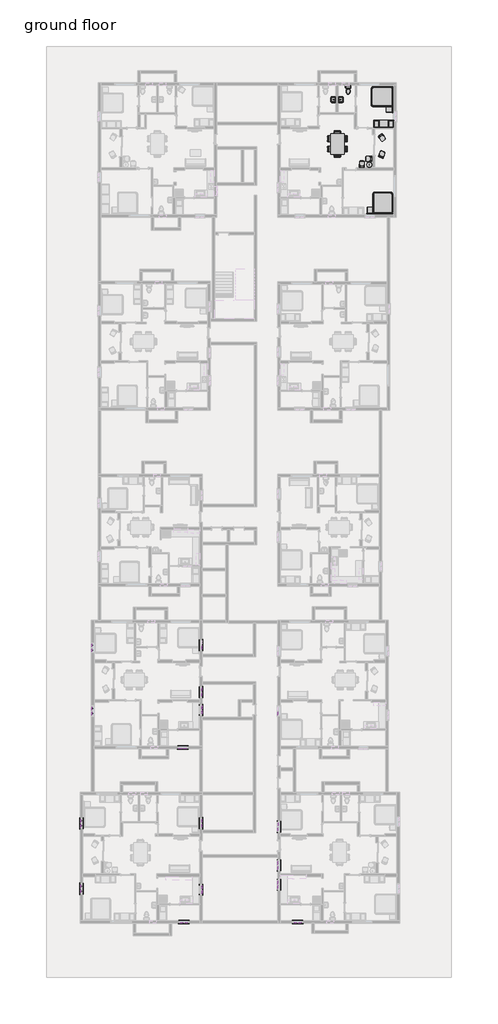
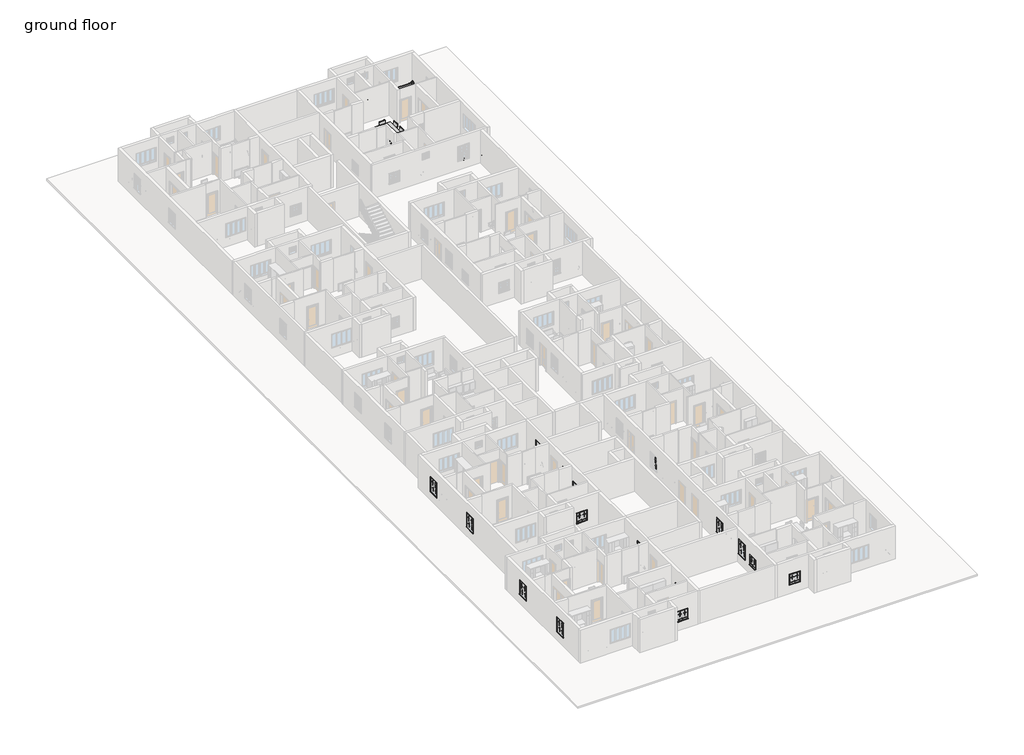
# One storey, part 14 of 16: 84 proxies, 15 furniture elements, 3 flow terminals.
"""IFC4 building model written with IfcOpenShell, lengths in millimetres."""

from ifc_helpers import new_model, si_unit, origin, place, context, project, spatial, transform, mapped, element, save
from components import muntin_pattern_2x2_muntin_pattern_2x2_cd1db81d, muntin_pattern_2x2_muntin_pattern_2x2_7c797e2d, muntin_pattern_2x2_muntin_pattern_2x2_78ce0566, muntin_pattern_2x2_muntin_pattern_2x2_27bf4e5b, muntin_pattern_2x2_muntin_pattern_2x2_8320156c, trim_window_exterior_flat_with_sill_fadbc092, trim_window_exterior_flat_with_sill_41619996, trim_window_interior_flat_picture_frame_db6fc9b7, trim_window_interior_flat_picture_frame_51c85655, flow_terminal_8d9ea526, toilet_domestic_3d_toilet_domestic_3d_ba6479b0, toilet_domestic_3d_toilet_domestic_3d_30431060, bed_design_8999_bed_design_8999_9c973422, bed_design_8999_bed_design_8999_e911dec7, chair_task_chair_task_b7f3823b, chair_task_arms_chair_task_arms_fa5a08ef, furniture_88072bd9, furniture_4fdbbe14, furniture_0bcc43ae, furniture_3dd5e188

model = new_model("IFC4")

# Units and contexts
model_context = context("Model", 3, world=origin())
ifc_project = project(units=[si_unit("LENGTHUNIT", "METRE", prefix="MILLI")], contexts=[model_context])

# Site, building, storey
site = spatial("IfcSite", under=ifc_project)
building = spatial("IfcBuilding", under=site)
storey = spatial("IfcBuildingStorey", under=building, Name="ground floor", Elevation=609.6)

# Proxies
placement = place(None, origin())
muntin_pattern_2x2_muntin_pattern_2x2_shape = muntin_pattern_2x2_muntin_pattern_2x2_cd1db81d(model_context)
element("IfcBuildingElementProxy", 1, Name="Muntin Pattern_2x2 : Muntin Pattern_2x2", ObjectType="Muntin Pattern_2x2 : Muntin Pattern_2x2", at=placement, inside=storey, context=model_context, shape_type="MappedRepresentation", body=[
    mapped(muntin_pattern_2x2_muntin_pattern_2x2_shape, transform((41563.651243, -22010.1303409, 2206.625), x_axis=(0.0, 1.0, 0.0), y_axis=(-1.0, 0.0, 0.0), z_axis=(0.0, 0.0, 1.0))),
])
element("IfcBuildingElementProxy", 2, Name="Muntin Pattern_2x2 : Muntin Pattern_2x2", ObjectType="Muntin Pattern_2x2 : Muntin Pattern_2x2", at=placement, inside=storey, context=model_context, shape_type="MappedRepresentation", body=[
    mapped(muntin_pattern_2x2_muntin_pattern_2x2_shape, transform((41608.101243, -22010.1303409, 1600.2), x_axis=(0.0, 1.0, 0.0), y_axis=(-1.0, 0.0, 0.0), z_axis=(0.0, 0.0, 1.0))),
])
element("IfcBuildingElementProxy", 3, Name="Muntin Pattern_2x2 : Muntin Pattern_2x2", ObjectType="Muntin Pattern_2x2 : Muntin Pattern_2x2", at=placement, inside=storey, context=model_context, shape_type="MappedRepresentation", body=[
    mapped(muntin_pattern_2x2_muntin_pattern_2x2_shape, transform((41563.651243, -16104.6303409, 2206.625), x_axis=(0.0, 1.0, 0.0), y_axis=(-1.0, 0.0, 0.0), z_axis=(0.0, 0.0, 1.0))),
])
element("IfcBuildingElementProxy", 4, Name="Muntin Pattern_2x2 : Muntin Pattern_2x2", ObjectType="Muntin Pattern_2x2 : Muntin Pattern_2x2", at=placement, inside=storey, context=model_context, shape_type="MappedRepresentation", body=[
    mapped(muntin_pattern_2x2_muntin_pattern_2x2_shape, transform((41608.101243, -16104.6303409, 1600.2), x_axis=(0.0, 1.0, 0.0), y_axis=(-1.0, 0.0, 0.0), z_axis=(0.0, 0.0, 1.0))),
])
element("IfcBuildingElementProxy", 5, Name="Muntin Pattern_2x2 : Muntin Pattern_2x2", ObjectType="Muntin Pattern_2x2 : Muntin Pattern_2x2", at=placement, inside=storey, context=model_context, shape_type="MappedRepresentation", body=[
    mapped(muntin_pattern_2x2_muntin_pattern_2x2_shape, transform((52504.701243, -16549.6721711, 2206.625), x_axis=(0.0, -1.0, 0.0), y_axis=(1.0, 0.0, 0.0), z_axis=(0.0, 0.0, 1.0))),
])
element("IfcBuildingElementProxy", 6, Name="Muntin Pattern_2x2 : Muntin Pattern_2x2", ObjectType="Muntin Pattern_2x2 : Muntin Pattern_2x2", at=placement, inside=storey, context=model_context, shape_type="MappedRepresentation", body=[
    mapped(muntin_pattern_2x2_muntin_pattern_2x2_shape, transform((52460.251243, -16549.6721711, 1600.2), x_axis=(0.0, -1.0, 0.0), y_axis=(1.0, 0.0, 0.0), z_axis=(0.0, 0.0, 1.0))),
])
element("IfcBuildingElementProxy", 7, Name="Muntin Pattern_2x2 : Muntin Pattern_2x2", ObjectType="Muntin Pattern_2x2 : Muntin Pattern_2x2", at=placement, inside=storey, context=model_context, shape_type="MappedRepresentation", body=[
    mapped(muntin_pattern_2x2_muntin_pattern_2x2_shape, transform((59391.4562819, -16409.4303409, 2206.625), x_axis=(0.0, 1.0, 0.0), y_axis=(-1.0, 0.0, 0.0), z_axis=(0.0, 0.0, 1.0))),
])
element("IfcBuildingElementProxy", 8, Name="Muntin Pattern_2x2 : Muntin Pattern_2x2", ObjectType="Muntin Pattern_2x2 : Muntin Pattern_2x2", at=placement, inside=storey, context=model_context, shape_type="MappedRepresentation", body=[
    mapped(muntin_pattern_2x2_muntin_pattern_2x2_shape, transform((59435.9062819, -16409.4303409, 1600.2), x_axis=(0.0, 1.0, 0.0), y_axis=(-1.0, 0.0, 0.0), z_axis=(0.0, 0.0, 1.0))),
])
element("IfcBuildingElementProxy", 9, Name="Muntin Pattern_2x2 : Muntin Pattern_2x2", ObjectType="Muntin Pattern_2x2 : Muntin Pattern_2x2", at=placement, inside=storey, context=model_context, shape_type="MappedRepresentation", body=[
    mapped(muntin_pattern_2x2_muntin_pattern_2x2_shape, transform((42566.951243, -5948.3051164, 2206.625), x_axis=(0.0, 1.0, 0.0), y_axis=(-1.0, 0.0, 0.0), z_axis=(0.0, 0.0, 1.0))),
])
element("IfcBuildingElementProxy", 10, Name="Muntin Pattern_2x2 : Muntin Pattern_2x2", ObjectType="Muntin Pattern_2x2 : Muntin Pattern_2x2", at=placement, inside=storey, context=model_context, shape_type="MappedRepresentation", body=[
    mapped(muntin_pattern_2x2_muntin_pattern_2x2_shape, transform((42611.401243, -5948.3051164, 1600.2), x_axis=(0.0, 1.0, 0.0), y_axis=(-1.0, 0.0, 0.0), z_axis=(0.0, 0.0, 1.0))),
])
element("IfcBuildingElementProxy", 11, Name="Muntin Pattern_2x2 : Muntin Pattern_2x2", ObjectType="Muntin Pattern_2x2 : Muntin Pattern_2x2", at=placement, inside=storey, context=model_context, shape_type="MappedRepresentation", body=[
    mapped(muntin_pattern_2x2_muntin_pattern_2x2_shape, transform((42566.951243, -233.3051164, 2206.625), x_axis=(0.0, 1.0, 0.0), y_axis=(-1.0, 0.0, 0.0), z_axis=(0.0, 0.0, 1.0))),
])
element("IfcBuildingElementProxy", 12, Name="Muntin Pattern_2x2 : Muntin Pattern_2x2", ObjectType="Muntin Pattern_2x2 : Muntin Pattern_2x2", at=placement, inside=storey, context=model_context, shape_type="MappedRepresentation", body=[
    mapped(muntin_pattern_2x2_muntin_pattern_2x2_shape, transform((42611.401243, -233.3051164, 1600.2), x_axis=(0.0, 1.0, 0.0), y_axis=(-1.0, 0.0, 0.0), z_axis=(0.0, 0.0, 1.0))),
])
element("IfcBuildingElementProxy", 13, Name="Muntin Pattern_2x2 : Muntin Pattern_2x2", ObjectType="Muntin Pattern_2x2 : Muntin Pattern_2x2", at=placement, inside=storey, context=model_context, shape_type="MappedRepresentation", body=[
    mapped(muntin_pattern_2x2_muntin_pattern_2x2_shape, transform((59391.4562819, -19899.7596399, 2206.625), x_axis=(0.0, 1.0, 0.0), y_axis=(-1.0, 0.0, 0.0), z_axis=(0.0, 0.0, 1.0))),
])
element("IfcBuildingElementProxy", 14, Name="Muntin Pattern_2x2 : Muntin Pattern_2x2", ObjectType="Muntin Pattern_2x2 : Muntin Pattern_2x2", at=placement, inside=storey, context=model_context, shape_type="MappedRepresentation", body=[
    mapped(muntin_pattern_2x2_muntin_pattern_2x2_shape, transform((59435.9062819, -19899.7596399, 1600.2), x_axis=(0.0, 1.0, 0.0), y_axis=(-1.0, 0.0, 0.0), z_axis=(0.0, 0.0, 1.0))),
])
element("IfcBuildingElementProxy", 15, Name="Muntin Pattern_2x2 : Muntin Pattern_2x2", ObjectType="Muntin Pattern_2x2 : Muntin Pattern_2x2", at=placement, inside=storey, context=model_context, shape_type="MappedRepresentation", body=[
    mapped(muntin_pattern_2x2_muntin_pattern_2x2_shape, transform((52504.701243, -4691.5814238, 2206.625), x_axis=(0.0, -1.0, 0.0), y_axis=(1.0, 0.0, 0.0), z_axis=(0.0, 0.0, 1.0))),
])
element("IfcBuildingElementProxy", 16, Name="Muntin Pattern_2x2 : Muntin Pattern_2x2", ObjectType="Muntin Pattern_2x2 : Muntin Pattern_2x2", at=placement, inside=storey, context=model_context, shape_type="MappedRepresentation", body=[
    mapped(muntin_pattern_2x2_muntin_pattern_2x2_shape, transform((52460.251243, -4691.5814238, 1600.2), x_axis=(0.0, -1.0, 0.0), y_axis=(1.0, 0.0, 0.0), z_axis=(0.0, 0.0, 1.0))),
])
element("IfcBuildingElementProxy", 17, Name="Muntin Pattern_2x2 : Muntin Pattern_2x2", ObjectType="Muntin Pattern_2x2 : Muntin Pattern_2x2", at=placement, inside=storey, context=model_context, shape_type="MappedRepresentation", body=[
    mapped(muntin_pattern_2x2_muntin_pattern_2x2_shape, transform((52504.701243, -452.6471815, 2206.625), x_axis=(0.0, -1.0, 0.0), y_axis=(1.0, 0.0, 0.0), z_axis=(0.0, 0.0, 1.0))),
])
element("IfcBuildingElementProxy", 18, Name="Muntin Pattern_2x2 : Muntin Pattern_2x2", ObjectType="Muntin Pattern_2x2 : Muntin Pattern_2x2", at=placement, inside=storey, context=model_context, shape_type="MappedRepresentation", body=[
    mapped(muntin_pattern_2x2_muntin_pattern_2x2_shape, transform((52460.251243, -452.6471815, 1600.2), x_axis=(0.0, -1.0, 0.0), y_axis=(1.0, 0.0, 0.0), z_axis=(0.0, 0.0, 1.0))),
])
muntin_pattern_2x2_muntin_pattern_2x2_2_shape = muntin_pattern_2x2_muntin_pattern_2x2_7c797e2d(model_context)
element("IfcBuildingElementProxy", 19, Name="Muntin Pattern_2x2 : Muntin Pattern_2x2", ObjectType="Muntin Pattern_2x2 : Muntin Pattern_2x2", at=placement, inside=storey, context=model_context, shape_type="MappedRepresentation", body=[
    mapped(muntin_pattern_2x2_muntin_pattern_2x2_2_shape, transform((59391.4562819, -6403.9176164, 2206.625), x_axis=(0.0, -1.0, 0.0), y_axis=(1.0, 0.0, 0.0), z_axis=(0.0, 0.0, 1.0))),
])
element("IfcBuildingElementProxy", 20, Name="Muntin Pattern_2x2 : Muntin Pattern_2x2", ObjectType="Muntin Pattern_2x2 : Muntin Pattern_2x2", at=placement, inside=storey, context=model_context, shape_type="MappedRepresentation", body=[
    mapped(muntin_pattern_2x2_muntin_pattern_2x2_2_shape, transform((59435.9062819, -6403.9176164, 1600.2), x_axis=(0.0, -1.0, 0.0), y_axis=(1.0, 0.0, 0.0), z_axis=(0.0, 0.0, 1.0))),
])
element("IfcBuildingElementProxy", 21, Name="Muntin Pattern_2x2 : Muntin Pattern_2x2", ObjectType="Muntin Pattern_2x2 : Muntin Pattern_2x2", at=placement, inside=storey, context=model_context, shape_type="MappedRepresentation", body=[
    mapped(muntin_pattern_2x2_muntin_pattern_2x2_2_shape, transform((41563.651243, -22465.7428409, 2206.625), x_axis=(0.0, -1.0, 0.0), y_axis=(1.0, 0.0, 0.0), z_axis=(0.0, 0.0, 1.0))),
])
element("IfcBuildingElementProxy", 22, Name="Muntin Pattern_2x2 : Muntin Pattern_2x2", ObjectType="Muntin Pattern_2x2 : Muntin Pattern_2x2", at=placement, inside=storey, context=model_context, shape_type="MappedRepresentation", body=[
    mapped(muntin_pattern_2x2_muntin_pattern_2x2_2_shape, transform((41608.101243, -22465.7428409, 1600.2), x_axis=(0.0, -1.0, 0.0), y_axis=(1.0, 0.0, 0.0), z_axis=(0.0, 0.0, 1.0))),
])
element("IfcBuildingElementProxy", 23, Name="Muntin Pattern_2x2 : Muntin Pattern_2x2", ObjectType="Muntin Pattern_2x2 : Muntin Pattern_2x2", at=placement, inside=storey, context=model_context, shape_type="MappedRepresentation", body=[
    mapped(muntin_pattern_2x2_muntin_pattern_2x2_2_shape, transform((41563.651243, -16560.2428409, 2206.625), x_axis=(0.0, -1.0, 0.0), y_axis=(1.0, 0.0, 0.0), z_axis=(0.0, 0.0, 1.0))),
])
element("IfcBuildingElementProxy", 24, Name="Muntin Pattern_2x2 : Muntin Pattern_2x2", ObjectType="Muntin Pattern_2x2 : Muntin Pattern_2x2", at=placement, inside=storey, context=model_context, shape_type="MappedRepresentation", body=[
    mapped(muntin_pattern_2x2_muntin_pattern_2x2_2_shape, transform((41608.101243, -16560.2428409, 1600.2), x_axis=(0.0, -1.0, 0.0), y_axis=(1.0, 0.0, 0.0), z_axis=(0.0, 0.0, 1.0))),
])
element("IfcBuildingElementProxy", 25, Name="Muntin Pattern_2x2 : Muntin Pattern_2x2", ObjectType="Muntin Pattern_2x2 : Muntin Pattern_2x2", at=placement, inside=storey, context=model_context, shape_type="MappedRepresentation", body=[
    mapped(muntin_pattern_2x2_muntin_pattern_2x2_2_shape, transform((52504.701243, -16094.0596711, 2206.625), x_axis=(0.0, 1.0, 0.0), y_axis=(-1.0, 0.0, 0.0), z_axis=(0.0, 0.0, 1.0))),
])
element("IfcBuildingElementProxy", 26, Name="Muntin Pattern_2x2 : Muntin Pattern_2x2", ObjectType="Muntin Pattern_2x2 : Muntin Pattern_2x2", at=placement, inside=storey, context=model_context, shape_type="MappedRepresentation", body=[
    mapped(muntin_pattern_2x2_muntin_pattern_2x2_2_shape, transform((52460.251243, -16094.0596711, 1600.2), x_axis=(0.0, 1.0, 0.0), y_axis=(-1.0, 0.0, 0.0), z_axis=(0.0, 0.0, 1.0))),
])
element("IfcBuildingElementProxy", 27, Name="Muntin Pattern_2x2 : Muntin Pattern_2x2", ObjectType="Muntin Pattern_2x2 : Muntin Pattern_2x2", at=placement, inside=storey, context=model_context, shape_type="MappedRepresentation", body=[
    mapped(muntin_pattern_2x2_muntin_pattern_2x2_2_shape, transform((59391.4562819, -16865.0428409, 2206.625), x_axis=(0.0, -1.0, 0.0), y_axis=(1.0, 0.0, 0.0), z_axis=(0.0, 0.0, 1.0))),
])
element("IfcBuildingElementProxy", 28, Name="Muntin Pattern_2x2 : Muntin Pattern_2x2", ObjectType="Muntin Pattern_2x2 : Muntin Pattern_2x2", at=placement, inside=storey, context=model_context, shape_type="MappedRepresentation", body=[
    mapped(muntin_pattern_2x2_muntin_pattern_2x2_2_shape, transform((59435.9062819, -16865.0428409, 1600.2), x_axis=(0.0, -1.0, 0.0), y_axis=(1.0, 0.0, 0.0), z_axis=(0.0, 0.0, 1.0))),
])
element("IfcBuildingElementProxy", 29, Name="Muntin Pattern_2x2 : Muntin Pattern_2x2", ObjectType="Muntin Pattern_2x2 : Muntin Pattern_2x2", at=placement, inside=storey, context=model_context, shape_type="MappedRepresentation", body=[
    mapped(muntin_pattern_2x2_muntin_pattern_2x2_2_shape, transform((42566.951243, -6403.9176164, 2206.625), x_axis=(0.0, -1.0, 0.0), y_axis=(1.0, 0.0, 0.0), z_axis=(0.0, 0.0, 1.0))),
])
element("IfcBuildingElementProxy", 30, Name="Muntin Pattern_2x2 : Muntin Pattern_2x2", ObjectType="Muntin Pattern_2x2 : Muntin Pattern_2x2", at=placement, inside=storey, context=model_context, shape_type="MappedRepresentation", body=[
    mapped(muntin_pattern_2x2_muntin_pattern_2x2_2_shape, transform((42611.401243, -6403.9176164, 1600.2), x_axis=(0.0, -1.0, 0.0), y_axis=(1.0, 0.0, 0.0), z_axis=(0.0, 0.0, 1.0))),
])
element("IfcBuildingElementProxy", 31, Name="Muntin Pattern_2x2 : Muntin Pattern_2x2", ObjectType="Muntin Pattern_2x2 : Muntin Pattern_2x2", at=placement, inside=storey, context=model_context, shape_type="MappedRepresentation", body=[
    mapped(muntin_pattern_2x2_muntin_pattern_2x2_2_shape, transform((42566.951243, -688.9176164, 2206.625), x_axis=(0.0, -1.0, 0.0), y_axis=(1.0, 0.0, 0.0), z_axis=(0.0, 0.0, 1.0))),
])
element("IfcBuildingElementProxy", 32, Name="Muntin Pattern_2x2 : Muntin Pattern_2x2", ObjectType="Muntin Pattern_2x2 : Muntin Pattern_2x2", at=placement, inside=storey, context=model_context, shape_type="MappedRepresentation", body=[
    mapped(muntin_pattern_2x2_muntin_pattern_2x2_2_shape, transform((42611.401243, -688.9176164, 1600.2), x_axis=(0.0, -1.0, 0.0), y_axis=(1.0, 0.0, 0.0), z_axis=(0.0, 0.0, 1.0))),
])
element("IfcBuildingElementProxy", 33, Name="Muntin Pattern_2x2 : Muntin Pattern_2x2", ObjectType="Muntin Pattern_2x2 : Muntin Pattern_2x2", at=placement, inside=storey, context=model_context, shape_type="MappedRepresentation", body=[
    mapped(muntin_pattern_2x2_muntin_pattern_2x2_2_shape, transform((59391.4562819, -20355.3721399, 2206.625), x_axis=(0.0, -1.0, 0.0), y_axis=(1.0, 0.0, 0.0), z_axis=(0.0, 0.0, 1.0))),
])
element("IfcBuildingElementProxy", 34, Name="Muntin Pattern_2x2 : Muntin Pattern_2x2", ObjectType="Muntin Pattern_2x2 : Muntin Pattern_2x2", at=placement, inside=storey, context=model_context, shape_type="MappedRepresentation", body=[
    mapped(muntin_pattern_2x2_muntin_pattern_2x2_2_shape, transform((59435.9062819, -20355.3721399, 1600.2), x_axis=(0.0, -1.0, 0.0), y_axis=(1.0, 0.0, 0.0), z_axis=(0.0, 0.0, 1.0))),
])
element("IfcBuildingElementProxy", 35, Name="Muntin Pattern_2x2 : Muntin Pattern_2x2", ObjectType="Muntin Pattern_2x2 : Muntin Pattern_2x2", at=placement, inside=storey, context=model_context, shape_type="MappedRepresentation", body=[
    mapped(muntin_pattern_2x2_muntin_pattern_2x2_2_shape, transform((52504.701243, -4235.9689238, 2206.625), x_axis=(0.0, 1.0, 0.0), y_axis=(-1.0, 0.0, 0.0), z_axis=(0.0, 0.0, 1.0))),
])
element("IfcBuildingElementProxy", 36, Name="Muntin Pattern_2x2 : Muntin Pattern_2x2", ObjectType="Muntin Pattern_2x2 : Muntin Pattern_2x2", at=placement, inside=storey, context=model_context, shape_type="MappedRepresentation", body=[
    mapped(muntin_pattern_2x2_muntin_pattern_2x2_2_shape, transform((52460.251243, -4235.9689238, 1600.2), x_axis=(0.0, 1.0, 0.0), y_axis=(-1.0, 0.0, 0.0), z_axis=(0.0, 0.0, 1.0))),
])
muntin_pattern_2x2_muntin_pattern_2x2_3_shape = muntin_pattern_2x2_muntin_pattern_2x2_78ce0566(model_context)
element("IfcBuildingElementProxy", 37, Name="Muntin Pattern_2x2 : Muntin Pattern_2x2", ObjectType="Muntin Pattern_2x2 : Muntin Pattern_2x2", at=placement, inside=storey, context=model_context, shape_type="MappedRepresentation", body=[
    mapped(muntin_pattern_2x2_muntin_pattern_2x2_3_shape, transform((59366.0562819, -22090.1783586, 1898.65), x_axis=(0.0, 1.0, 0.0), y_axis=(-1.0, 0.0, 0.0), z_axis=(0.0, 0.0, 1.0))),
])
element("IfcBuildingElementProxy", 38, Name="Muntin Pattern_2x2 : Muntin Pattern_2x2", ObjectType="Muntin Pattern_2x2 : Muntin Pattern_2x2", at=placement, inside=storey, context=model_context, shape_type="MappedRepresentation", body=[
    mapped(muntin_pattern_2x2_muntin_pattern_2x2_3_shape, transform((61376.3046849, -25339.9115909, 1898.65), x_axis=(-1.0, 0.0, 0.0), y_axis=(0.0, -1.0, 0.0), z_axis=(0.0, 0.0, 1.0))),
])
element("IfcBuildingElementProxy", 39, Name="Muntin Pattern_2x2 : Muntin Pattern_2x2", ObjectType="Muntin Pattern_2x2 : Muntin Pattern_2x2", at=placement, inside=storey, context=model_context, shape_type="MappedRepresentation", body=[
    mapped(muntin_pattern_2x2_muntin_pattern_2x2_3_shape, transform((51095.820268, -25339.9115909, 1898.65), x_axis=(-1.0, 0.0, 0.0), y_axis=(0.0, -1.0, 0.0), z_axis=(0.0, 0.0, 1.0))),
])
element("IfcBuildingElementProxy", 40, Name="Muntin Pattern_2x2 : Muntin Pattern_2x2", ObjectType="Muntin Pattern_2x2 : Muntin Pattern_2x2", at=placement, inside=storey, context=model_context, shape_type="MappedRepresentation", body=[
    mapped(muntin_pattern_2x2_muntin_pattern_2x2_3_shape, transform((52530.101243, -22109.3490909, 1898.65), x_axis=(0.0, -1.0, 0.0), y_axis=(1.0, 0.0, 0.0), z_axis=(0.0, 0.0, 1.0))),
])
element("IfcBuildingElementProxy", 41, Name="Muntin Pattern_2x2 : Muntin Pattern_2x2", ObjectType="Muntin Pattern_2x2 : Muntin Pattern_2x2", at=placement, inside=storey, context=model_context, shape_type="MappedRepresentation", body=[
    mapped(muntin_pattern_2x2_muntin_pattern_2x2_3_shape, transform((51000.4634253, -9576.8003443, 1898.65), x_axis=(-1.0, 0.0, 0.0), y_axis=(0.0, -1.0, 0.0), z_axis=(0.0, 0.0, 1.0))),
])
element("IfcBuildingElementProxy", 42, Name="Muntin Pattern_2x2 : Muntin Pattern_2x2", ObjectType="Muntin Pattern_2x2 : Muntin Pattern_2x2", at=placement, inside=storey, context=model_context, shape_type="MappedRepresentation", body=[
    mapped(muntin_pattern_2x2_muntin_pattern_2x2_3_shape, transform((52530.101243, -5866.8447725, 1898.65), x_axis=(0.0, -1.0, 0.0), y_axis=(1.0, 0.0, 0.0), z_axis=(0.0, 0.0, 1.0))),
])
muntin_pattern_2x2_muntin_pattern_2x2_4_shape = muntin_pattern_2x2_muntin_pattern_2x2_27bf4e5b(model_context)
element("IfcBuildingElementProxy", 43, Name="Muntin Pattern_2x2 : Muntin Pattern_2x2", ObjectType="Muntin Pattern_2x2 : Muntin Pattern_2x2", at=placement, inside=storey, context=model_context, shape_type="MappedRepresentation", body=[
    mapped(muntin_pattern_2x2_muntin_pattern_2x2_4_shape, transform((59366.0562819, -21661.5533586, 1898.65), x_axis=(0.0, -1.0, 0.0), y_axis=(1.0, 0.0, 0.0), z_axis=(0.0, 0.0, 1.0))),
])
element("IfcBuildingElementProxy", 44, Name="Muntin Pattern_2x2 : Muntin Pattern_2x2", ObjectType="Muntin Pattern_2x2 : Muntin Pattern_2x2", at=placement, inside=storey, context=model_context, shape_type="MappedRepresentation", body=[
    mapped(muntin_pattern_2x2_muntin_pattern_2x2_4_shape, transform((60947.6796849, -25339.9115909, 1898.65), x_axis=(1.0, 0.0, 0.0), y_axis=(0.0, 1.0, 0.0), z_axis=(0.0, 0.0, 1.0))),
])
element("IfcBuildingElementProxy", 45, Name="Muntin Pattern_2x2 : Muntin Pattern_2x2", ObjectType="Muntin Pattern_2x2 : Muntin Pattern_2x2", at=placement, inside=storey, context=model_context, shape_type="MappedRepresentation", body=[
    mapped(muntin_pattern_2x2_muntin_pattern_2x2_4_shape, transform((50667.195268, -25339.9115909, 1898.65), x_axis=(1.0, 0.0, 0.0), y_axis=(0.0, 1.0, 0.0), z_axis=(0.0, 0.0, 1.0))),
])
element("IfcBuildingElementProxy", 46, Name="Muntin Pattern_2x2 : Muntin Pattern_2x2", ObjectType="Muntin Pattern_2x2 : Muntin Pattern_2x2", at=placement, inside=storey, context=model_context, shape_type="MappedRepresentation", body=[
    mapped(muntin_pattern_2x2_muntin_pattern_2x2_4_shape, transform((52530.101243, -22537.9740909, 1898.65), x_axis=(0.0, 1.0, 0.0), y_axis=(-1.0, 0.0, 0.0), z_axis=(0.0, 0.0, 1.0))),
])
element("IfcBuildingElementProxy", 47, Name="Muntin Pattern_2x2 : Muntin Pattern_2x2", ObjectType="Muntin Pattern_2x2 : Muntin Pattern_2x2", at=placement, inside=storey, context=model_context, shape_type="MappedRepresentation", body=[
    mapped(muntin_pattern_2x2_muntin_pattern_2x2_4_shape, transform((50571.8384253, -9576.8003443, 1898.65), x_axis=(1.0, 0.0, 0.0), y_axis=(0.0, 1.0, 0.0), z_axis=(0.0, 0.0, 1.0))),
])
element("IfcBuildingElementProxy", 48, Name="Muntin Pattern_2x2 : Muntin Pattern_2x2", ObjectType="Muntin Pattern_2x2 : Muntin Pattern_2x2", at=placement, inside=storey, context=model_context, shape_type="MappedRepresentation", body=[
    mapped(muntin_pattern_2x2_muntin_pattern_2x2_4_shape, transform((52530.101243, -6295.4697725, 1898.65), x_axis=(0.0, 1.0, 0.0), y_axis=(-1.0, 0.0, 0.0), z_axis=(0.0, 0.0, 1.0))),
])
muntin_pattern_2x2_muntin_pattern_2x2_5_shape = muntin_pattern_2x2_muntin_pattern_2x2_8320156c(model_context)
element("IfcBuildingElementProxy", 49, Name="Muntin Pattern_2x2 : Muntin Pattern_2x2", ObjectType="Muntin Pattern_2x2 : Muntin Pattern_2x2", at=placement, inside=storey, context=model_context, shape_type="MappedRepresentation", body=[
    mapped(muntin_pattern_2x2_muntin_pattern_2x2_5_shape, transform((59366.0562819, -21875.8658586, 1593.85), x_axis=(0.0, -1.0, 0.0), y_axis=(1.0, 0.0, 0.0), z_axis=(0.0, 0.0, 1.0))),
])
element("IfcBuildingElementProxy", 50, Name="Muntin Pattern_2x2 : Muntin Pattern_2x2", ObjectType="Muntin Pattern_2x2 : Muntin Pattern_2x2", at=placement, inside=storey, context=model_context, shape_type="MappedRepresentation", body=[
    mapped(muntin_pattern_2x2_muntin_pattern_2x2_5_shape, transform((61161.9921849, -25339.9115909, 1593.85), x_axis=(1.0, 0.0, 0.0), y_axis=(0.0, 1.0, 0.0), z_axis=(0.0, 0.0, 1.0))),
])
element("IfcBuildingElementProxy", 51, Name="Muntin Pattern_2x2 : Muntin Pattern_2x2", ObjectType="Muntin Pattern_2x2 : Muntin Pattern_2x2", at=placement, inside=storey, context=model_context, shape_type="MappedRepresentation", body=[
    mapped(muntin_pattern_2x2_muntin_pattern_2x2_5_shape, transform((50881.507768, -25339.9115909, 1593.85), x_axis=(1.0, 0.0, 0.0), y_axis=(0.0, 1.0, 0.0), z_axis=(0.0, 0.0, 1.0))),
])
element("IfcBuildingElementProxy", 52, Name="Muntin Pattern_2x2 : Muntin Pattern_2x2", ObjectType="Muntin Pattern_2x2 : Muntin Pattern_2x2", at=placement, inside=storey, context=model_context, shape_type="MappedRepresentation", body=[
    mapped(muntin_pattern_2x2_muntin_pattern_2x2_5_shape, transform((52530.101243, -22323.6615909, 1593.85), x_axis=(0.0, 1.0, 0.0), y_axis=(-1.0, 0.0, 0.0), z_axis=(0.0, 0.0, 1.0))),
])
element("IfcBuildingElementProxy", 53, Name="Muntin Pattern_2x2 : Muntin Pattern_2x2", ObjectType="Muntin Pattern_2x2 : Muntin Pattern_2x2", at=placement, inside=storey, context=model_context, shape_type="MappedRepresentation", body=[
    mapped(muntin_pattern_2x2_muntin_pattern_2x2_5_shape, transform((50786.1509253, -9576.8003443, 1593.85), x_axis=(1.0, 0.0, 0.0), y_axis=(0.0, 1.0, 0.0), z_axis=(0.0, 0.0, 1.0))),
])
element("IfcBuildingElementProxy", 54, Name="Muntin Pattern_2x2 : Muntin Pattern_2x2", ObjectType="Muntin Pattern_2x2 : Muntin Pattern_2x2", at=placement, inside=storey, context=model_context, shape_type="MappedRepresentation", body=[
    mapped(muntin_pattern_2x2_muntin_pattern_2x2_5_shape, transform((52530.101243, -6081.1572725, 1593.85), x_axis=(0.0, 1.0, 0.0), y_axis=(-1.0, 0.0, 0.0), z_axis=(0.0, 0.0, 1.0))),
])
trim_window_exterior_flat_with_sill_shape = trim_window_exterior_flat_with_sill_fadbc092(model_context)
element("IfcBuildingElementProxy", 55, Name="Trim-Window-Exterior-Flat : with Sill", ObjectType="Trim-Window-Exterior-Flat : with Sill", at=placement, inside=storey, context=model_context, shape_type="MappedRepresentation", body=[
    mapped(trim_window_exterior_flat_with_sill_shape, transform((41528.726243, -22237.9365909, 2844.8), x_axis=(0.0, -1.0, 0.0), y_axis=(0.0, 0.0, 1.0), z_axis=(-1.0, 0.0, 0.0))),
])
element("IfcBuildingElementProxy", 56, Name="Trim-Window-Exterior-Flat : with Sill", ObjectType="Trim-Window-Exterior-Flat : with Sill", at=placement, inside=storey, context=model_context, shape_type="MappedRepresentation", body=[
    mapped(trim_window_exterior_flat_with_sill_shape, transform((41528.726243, -16332.4365909, 2844.8), x_axis=(0.0, -1.0, 0.0), y_axis=(0.0, 0.0, 1.0), z_axis=(-1.0, 0.0, 0.0))),
])
element("IfcBuildingElementProxy", 57, Name="Trim-Window-Exterior-Flat : with Sill", ObjectType="Trim-Window-Exterior-Flat : with Sill", at=placement, inside=storey, context=model_context, shape_type="MappedRepresentation", body=[
    mapped(trim_window_exterior_flat_with_sill_shape, transform((52539.626243, -16321.8659211, 2844.8), x_axis=(0.0, 1.0, 0.0), y_axis=(0.0, 0.0, 1.0), z_axis=(1.0, 0.0, 0.0))),
])
element("IfcBuildingElementProxy", 58, Name="Trim-Window-Exterior-Flat : with Sill", ObjectType="Trim-Window-Exterior-Flat : with Sill", at=placement, inside=storey, context=model_context, shape_type="MappedRepresentation", body=[
    mapped(trim_window_exterior_flat_with_sill_shape, transform((59356.5312819, -16637.2365909, 2844.8), x_axis=(0.0, -1.0, 0.0), y_axis=(0.0, 0.0, 1.0), z_axis=(-1.0, 0.0, 0.0))),
])
element("IfcBuildingElementProxy", 59, Name="Trim-Window-Exterior-Flat : with Sill", ObjectType="Trim-Window-Exterior-Flat : with Sill", at=placement, inside=storey, context=model_context, shape_type="MappedRepresentation", body=[
    mapped(trim_window_exterior_flat_with_sill_shape, transform((42532.026243, -6176.1113664, 2844.8), x_axis=(0.0, -1.0, 0.0), y_axis=(0.0, 0.0, 1.0), z_axis=(-1.0, 0.0, 0.0))),
])
element("IfcBuildingElementProxy", 60, Name="Trim-Window-Exterior-Flat : with Sill", ObjectType="Trim-Window-Exterior-Flat : with Sill", at=placement, inside=storey, context=model_context, shape_type="MappedRepresentation", body=[
    mapped(trim_window_exterior_flat_with_sill_shape, transform((42532.026243, -461.1113664, 2844.8), x_axis=(0.0, -1.0, 0.0), y_axis=(0.0, 0.0, 1.0), z_axis=(-1.0, 0.0, 0.0))),
])
element("IfcBuildingElementProxy", 61, Name="Trim-Window-Exterior-Flat : with Sill", ObjectType="Trim-Window-Exterior-Flat : with Sill", at=placement, inside=storey, context=model_context, shape_type="MappedRepresentation", body=[
    mapped(trim_window_exterior_flat_with_sill_shape, transform((59356.5312819, -20127.5658899, 2844.8), x_axis=(0.0, -1.0, 0.0), y_axis=(0.0, 0.0, 1.0), z_axis=(-1.0, 0.0, 0.0))),
])
element("IfcBuildingElementProxy", 62, Name="Trim-Window-Exterior-Flat : with Sill", ObjectType="Trim-Window-Exterior-Flat : with Sill", at=placement, inside=storey, context=model_context, shape_type="MappedRepresentation", body=[
    mapped(trim_window_exterior_flat_with_sill_shape, transform((52539.626243, -4463.7751738, 2844.8), x_axis=(0.0, 1.0, 0.0), y_axis=(0.0, 0.0, 1.0), z_axis=(1.0, 0.0, 0.0))),
])
element("IfcBuildingElementProxy", 63, Name="Trim-Window-Exterior-Flat : with Sill", ObjectType="Trim-Window-Exterior-Flat : with Sill", at=placement, inside=storey, context=model_context, shape_type="MappedRepresentation", body=[
    mapped(trim_window_exterior_flat_with_sill_shape, transform((52539.626243, -224.8409315, 2844.8), x_axis=(0.0, 1.0, 0.0), y_axis=(0.0, 0.0, 1.0), z_axis=(1.0, 0.0, 0.0))),
])
trim_window_exterior_flat_with_sill_2_shape = trim_window_exterior_flat_with_sill_41619996(model_context)
element("IfcBuildingElementProxy", 64, Name="Trim-Window-Exterior-Flat : with Sill", ObjectType="Trim-Window-Exterior-Flat : with Sill", at=placement, inside=storey, context=model_context, shape_type="MappedRepresentation", body=[
    mapped(trim_window_exterior_flat_with_sill_2_shape, transform((59356.5312819, -21875.8658586, 2438.4), x_axis=(0.0, -1.0, 0.0), y_axis=(0.0, 0.0, 1.0), z_axis=(-1.0, 0.0, 0.0))),
])
element("IfcBuildingElementProxy", 65, Name="Trim-Window-Exterior-Flat : with Sill", ObjectType="Trim-Window-Exterior-Flat : with Sill", at=placement, inside=storey, context=model_context, shape_type="MappedRepresentation", body=[
    mapped(trim_window_exterior_flat_with_sill_2_shape, transform((61161.9921849, -25349.4365909, 2438.4), x_axis=(1.0, 0.0, 0.0), y_axis=(0.0, 0.0, 1.0), z_axis=(0.0, -1.0, 0.0))),
])
element("IfcBuildingElementProxy", 66, Name="Trim-Window-Exterior-Flat : with Sill", ObjectType="Trim-Window-Exterior-Flat : with Sill", at=placement, inside=storey, context=model_context, shape_type="MappedRepresentation", body=[
    mapped(trim_window_exterior_flat_with_sill_2_shape, transform((50881.507768, -25349.4365909, 2438.4), x_axis=(1.0, 0.0, 0.0), y_axis=(0.0, 0.0, 1.0), z_axis=(0.0, -1.0, 0.0))),
])
element("IfcBuildingElementProxy", 67, Name="Trim-Window-Exterior-Flat : with Sill", ObjectType="Trim-Window-Exterior-Flat : with Sill", at=placement, inside=storey, context=model_context, shape_type="MappedRepresentation", body=[
    mapped(trim_window_exterior_flat_with_sill_2_shape, transform((52539.626243, -22323.6615909, 2438.4), x_axis=(0.0, 1.0, 0.0), y_axis=(0.0, 0.0, 1.0), z_axis=(1.0, 0.0, 0.0))),
])
element("IfcBuildingElementProxy", 68, Name="Trim-Window-Exterior-Flat : with Sill", ObjectType="Trim-Window-Exterior-Flat : with Sill", at=placement, inside=storey, context=model_context, shape_type="MappedRepresentation", body=[
    mapped(trim_window_exterior_flat_with_sill_2_shape, transform((50786.1509253, -9586.3253443, 2438.4), x_axis=(1.0, 0.0, 0.0), y_axis=(0.0, 0.0, 1.0), z_axis=(0.0, -1.0, 0.0))),
])
element("IfcBuildingElementProxy", 69, Name="Trim-Window-Exterior-Flat : with Sill", ObjectType="Trim-Window-Exterior-Flat : with Sill", at=placement, inside=storey, context=model_context, shape_type="MappedRepresentation", body=[
    mapped(trim_window_exterior_flat_with_sill_2_shape, transform((52539.626243, -6081.1572725, 2438.4), x_axis=(0.0, 1.0, 0.0), y_axis=(0.0, 0.0, 1.0), z_axis=(1.0, 0.0, 0.0))),
])
trim_window_interior_flat_picture_frame_shape = trim_window_interior_flat_picture_frame_db6fc9b7(model_context)
element("IfcBuildingElementProxy", 70, Name="Trim-Window-Interior-Flat : Picture Frame", ObjectType="Trim-Window-Interior-Flat : Picture Frame", at=placement, inside=storey, context=model_context, shape_type="MappedRepresentation", body=[
    mapped(trim_window_interior_flat_picture_frame_shape, transform((41757.326243, -22237.9365909, 2844.8), x_axis=(0.0, 1.0, 0.0), y_axis=(0.0, 0.0, 1.0), z_axis=(1.0, 0.0, 0.0))),
])
element("IfcBuildingElementProxy", 71, Name="Trim-Window-Interior-Flat : Picture Frame", ObjectType="Trim-Window-Interior-Flat : Picture Frame", at=placement, inside=storey, context=model_context, shape_type="MappedRepresentation", body=[
    mapped(trim_window_interior_flat_picture_frame_shape, transform((41757.326243, -16332.4365909, 2844.8), x_axis=(0.0, 1.0, 0.0), y_axis=(0.0, 0.0, 1.0), z_axis=(1.0, 0.0, 0.0))),
])
element("IfcBuildingElementProxy", 72, Name="Trim-Window-Interior-Flat : Picture Frame", ObjectType="Trim-Window-Interior-Flat : Picture Frame", at=placement, inside=storey, context=model_context, shape_type="MappedRepresentation", body=[
    mapped(trim_window_interior_flat_picture_frame_shape, transform((52311.026243, -16321.8659211, 2844.8), x_axis=(0.0, -1.0, 0.0), y_axis=(0.0, 0.0, 1.0), z_axis=(-1.0, 0.0, 0.0))),
])
element("IfcBuildingElementProxy", 73, Name="Trim-Window-Interior-Flat : Picture Frame", ObjectType="Trim-Window-Interior-Flat : Picture Frame", at=placement, inside=storey, context=model_context, shape_type="MappedRepresentation", body=[
    mapped(trim_window_interior_flat_picture_frame_shape, transform((59585.1312819, -16637.2365909, 2844.8), x_axis=(0.0, 1.0, 0.0), y_axis=(0.0, 0.0, 1.0), z_axis=(1.0, 0.0, 0.0))),
])
element("IfcBuildingElementProxy", 74, Name="Trim-Window-Interior-Flat : Picture Frame", ObjectType="Trim-Window-Interior-Flat : Picture Frame", at=placement, inside=storey, context=model_context, shape_type="MappedRepresentation", body=[
    mapped(trim_window_interior_flat_picture_frame_shape, transform((42760.626243, -6176.1113664, 2844.8), x_axis=(0.0, 1.0, 0.0), y_axis=(0.0, 0.0, 1.0), z_axis=(1.0, 0.0, 0.0))),
])
element("IfcBuildingElementProxy", 75, Name="Trim-Window-Interior-Flat : Picture Frame", ObjectType="Trim-Window-Interior-Flat : Picture Frame", at=placement, inside=storey, context=model_context, shape_type="MappedRepresentation", body=[
    mapped(trim_window_interior_flat_picture_frame_shape, transform((42760.626243, -461.1113664, 2844.8), x_axis=(0.0, 1.0, 0.0), y_axis=(0.0, 0.0, 1.0), z_axis=(1.0, 0.0, 0.0))),
])
element("IfcBuildingElementProxy", 76, Name="Trim-Window-Interior-Flat : Picture Frame", ObjectType="Trim-Window-Interior-Flat : Picture Frame", at=placement, inside=storey, context=model_context, shape_type="MappedRepresentation", body=[
    mapped(trim_window_interior_flat_picture_frame_shape, transform((59585.1312819, -20127.5658899, 2844.8), x_axis=(0.0, 1.0, 0.0), y_axis=(0.0, 0.0, 1.0), z_axis=(1.0, 0.0, 0.0))),
])
element("IfcBuildingElementProxy", 77, Name="Trim-Window-Interior-Flat : Picture Frame", ObjectType="Trim-Window-Interior-Flat : Picture Frame", at=placement, inside=storey, context=model_context, shape_type="MappedRepresentation", body=[
    mapped(trim_window_interior_flat_picture_frame_shape, transform((52311.026243, -4463.7751738, 2844.8), x_axis=(0.0, -1.0, 0.0), y_axis=(0.0, 0.0, 1.0), z_axis=(-1.0, 0.0, 0.0))),
])
element("IfcBuildingElementProxy", 78, Name="Trim-Window-Interior-Flat : Picture Frame", ObjectType="Trim-Window-Interior-Flat : Picture Frame", at=placement, inside=storey, context=model_context, shape_type="MappedRepresentation", body=[
    mapped(trim_window_interior_flat_picture_frame_shape, transform((52311.026243, -224.8409315, 2844.8), x_axis=(0.0, -1.0, 0.0), y_axis=(0.0, 0.0, 1.0), z_axis=(-1.0, 0.0, 0.0))),
])
trim_window_interior_flat_picture_frame_2_shape = trim_window_interior_flat_picture_frame_51c85655(model_context)
element("IfcBuildingElementProxy", 79, Name="Trim-Window-Interior-Flat : Picture Frame", ObjectType="Trim-Window-Interior-Flat : Picture Frame", at=placement, inside=storey, context=model_context, shape_type="MappedRepresentation", body=[
    mapped(trim_window_interior_flat_picture_frame_2_shape, transform((59585.1312819, -21875.8658586, 2438.4), x_axis=(0.0, 1.0, 0.0), y_axis=(0.0, 0.0, 1.0), z_axis=(1.0, 0.0, 0.0))),
])
element("IfcBuildingElementProxy", 80, Name="Trim-Window-Interior-Flat : Picture Frame", ObjectType="Trim-Window-Interior-Flat : Picture Frame", at=placement, inside=storey, context=model_context, shape_type="MappedRepresentation", body=[
    mapped(trim_window_interior_flat_picture_frame_2_shape, transform((61161.9921849, -25120.8365909, 2438.4), x_axis=(-1.0, 0.0, 0.0), y_axis=(0.0, 0.0, 1.0), z_axis=(0.0, 1.0, 0.0))),
])
element("IfcBuildingElementProxy", 81, Name="Trim-Window-Interior-Flat : Picture Frame", ObjectType="Trim-Window-Interior-Flat : Picture Frame", at=placement, inside=storey, context=model_context, shape_type="MappedRepresentation", body=[
    mapped(trim_window_interior_flat_picture_frame_2_shape, transform((50881.507768, -25120.8365909, 2438.4), x_axis=(-1.0, 0.0, 0.0), y_axis=(0.0, 0.0, 1.0), z_axis=(0.0, 1.0, 0.0))),
])
element("IfcBuildingElementProxy", 82, Name="Trim-Window-Interior-Flat : Picture Frame", ObjectType="Trim-Window-Interior-Flat : Picture Frame", at=placement, inside=storey, context=model_context, shape_type="MappedRepresentation", body=[
    mapped(trim_window_interior_flat_picture_frame_2_shape, transform((52311.026243, -22323.6615909, 2438.4), x_axis=(0.0, -1.0, 0.0), y_axis=(0.0, 0.0, 1.0), z_axis=(-1.0, 0.0, 0.0))),
])
element("IfcBuildingElementProxy", 83, Name="Trim-Window-Interior-Flat : Picture Frame", ObjectType="Trim-Window-Interior-Flat : Picture Frame", at=placement, inside=storey, context=model_context, shape_type="MappedRepresentation", body=[
    mapped(trim_window_interior_flat_picture_frame_2_shape, transform((50786.1509253, -9357.7253443, 2438.4), x_axis=(-1.0, 0.0, 0.0), y_axis=(0.0, 0.0, 1.0), z_axis=(0.0, 1.0, 0.0))),
])
element("IfcBuildingElementProxy", 84, Name="Trim-Window-Interior-Flat : Picture Frame", ObjectType="Trim-Window-Interior-Flat : Picture Frame", at=placement, inside=storey, context=model_context, shape_type="MappedRepresentation", body=[
    mapped(trim_window_interior_flat_picture_frame_2_shape, transform((52311.026243, -6081.1572725, 2438.4), x_axis=(0.0, -1.0, 0.0), y_axis=(0.0, 0.0, 1.0), z_axis=(-1.0, 0.0, 0.0))),
])

# Flow terminals
flow_terminal_shape = flow_terminal_8d9ea526(model_context)
element("IfcFlowTerminal", 85, ObjectType="Sink Vanity-Square : 20\" x 18\"", at=placement, inside=storey, context=model_context, shape_type="MappedRepresentation", body=[
    mapped(flow_terminal_shape, transform((65002.967982, 49049.8022203, 609.6), x_axis=(0.0, 1.0, 0.0), y_axis=(-1.0, 0.0, 0.0), z_axis=(0.0, 0.0, 1.0))),
])
element("IfcFlowTerminal", 86, ObjectType="Sink Vanity-Square : 20\" x 18\"", at=placement, inside=storey, context=model_context, shape_type="MappedRepresentation", body=[
    mapped(flow_terminal_shape, transform((64438.6417871, 49081.1807014, 609.6), x_axis=(0.0, -1.0, 0.0), y_axis=(1.0, 0.0, 0.0), z_axis=(0.0, 0.0, 1.0))),
])
toilet_domestic_3d_toilet_domestic_3d_shape = toilet_domestic_3d_toilet_domestic_3d_ba6479b0(model_context)
toilet_domestic_3d_toilet_domestic_3d_2_shape = toilet_domestic_3d_toilet_domestic_3d_30431060(model_context)
element("IfcFlowTerminal", 87, ObjectType="Toilet-Domestic-3D : Toilet-Domestic-3D", at=placement, inside=storey, context=model_context, shape_type="MappedRepresentation", body=[
    mapped(toilet_domestic_3d_toilet_domestic_3d_shape, transform((65726.0226571, 49859.7430562, 609.6), x_axis=(1.0, 0.0, 0.0), y_axis=(0.0, 1.0, 0.0), z_axis=(0.0, 0.0, 1.0))),
    mapped(toilet_domestic_3d_toilet_domestic_3d_2_shape, transform((65726.0226571, 49859.7430562, 609.6), x_axis=(1.0, 0.0, 0.0), y_axis=(0.0, 1.0, 0.0), z_axis=(0.0, 0.0, 1.0))),
])

# Furniture
bed_design_8999_bed_design_8999_shape = bed_design_8999_bed_design_8999_9c973422(model_context)
bed_design_8999_bed_design_8999_2_shape = bed_design_8999_bed_design_8999_e911dec7(model_context)
element("IfcFurniture", 88, ObjectType="BED_DESIGN_8999 : BED_DESIGN_8999", at=placement, inside=storey, context=model_context, shape_type="MappedRepresentation", body=[
    mapped(bed_design_8999_bed_design_8999_shape, transform((67804.1945107, 49137.2273256, 609.6), x_axis=(0.0, -1.0, 0.0), y_axis=(1.0, 0.0, 0.0), z_axis=(0.0, 0.0, 1.0))),
    mapped(bed_design_8999_bed_design_8999_2_shape, transform((67804.1945107, 49137.2273256, 609.6), x_axis=(0.0, -1.0, 0.0), y_axis=(1.0, 0.0, 0.0), z_axis=(0.0, 0.0, 1.0))),
])
element("IfcFurniture", 89, ObjectType="BED_DESIGN_8999 : BED_DESIGN_8999", at=placement, inside=storey, context=model_context, shape_type="MappedRepresentation", body=[
    mapped(bed_design_8999_bed_design_8999_shape, transform((68657.3757323, 40719.5817487, 609.6), x_axis=(-1.0, 0.0, 0.0), y_axis=(0.0, -1.0, 0.0), z_axis=(0.0, 0.0, 1.0))),
    mapped(bed_design_8999_bed_design_8999_2_shape, transform((68657.3757323, 40719.5817487, 609.6), x_axis=(-1.0, 0.0, 0.0), y_axis=(0.0, -1.0, 0.0), z_axis=(0.0, 0.0, 1.0))),
])
chair_task_chair_task_shape = chair_task_chair_task_b7f3823b(model_context)
element("IfcFurniture", 90, ObjectType="Chair-Task : Chair-Task", at=placement, inside=storey, context=model_context, shape_type="MappedRepresentation", body=[
    mapped(chair_task_chair_task_shape, transform((64118.5297305, 45663.0104868, 609.6), x_axis=(0.0, -1.0, 0.0), y_axis=(1.0, 0.0, 0.0), z_axis=(0.0, 0.0, 1.0))),
])
element("IfcFurniture", 91, ObjectType="Chair-Task : Chair-Task", at=placement, inside=storey, context=model_context, shape_type="MappedRepresentation", body=[
    mapped(chair_task_chair_task_shape, transform((65375.6215338, 45381.0288474, 609.6), x_axis=(0.0, 1.0, 0.0), y_axis=(-1.0, 0.0, 0.0), z_axis=(0.0, 0.0, 1.0))),
])
element("IfcFurniture", 92, ObjectType="Chair-Task : Chair-Task", at=placement, inside=storey, context=model_context, shape_type="MappedRepresentation", body=[
    mapped(chair_task_chair_task_shape, transform((64118.5297305, 44748.6104868, 609.6), x_axis=(0.0, -1.0, 0.0), y_axis=(1.0, 0.0, 0.0), z_axis=(0.0, 0.0, 1.0))),
])
element("IfcFurniture", 93, ObjectType="Chair-Task : Chair-Task", at=placement, inside=storey, context=model_context, shape_type="MappedRepresentation", body=[
    mapped(chair_task_chair_task_shape, transform((65375.6215338, 44466.6288474, 609.6), x_axis=(0.0, 1.0, 0.0), y_axis=(-1.0, 0.0, 0.0), z_axis=(0.0, 0.0, 1.0))),
])
chair_task_arms_chair_task_arms_shape = chair_task_arms_chair_task_arms_fa5a08ef(model_context)
element("IfcFurniture", 94, ObjectType="Chair-Task Arms : Chair-Task Arms", at=placement, inside=storey, context=model_context, shape_type="MappedRepresentation", body=[
    mapped(chair_task_arms_chair_task_arms_shape, transform((64606.0848124, 44131.4737655, 609.6), x_axis=(1.0, 0.0, 0.0), y_axis=(0.0, 1.0, 0.0), z_axis=(0.0, 0.0, 1.0))),
])
element("IfcFurniture", 95, ObjectType="Chair-Task Arms : Chair-Task Arms", at=placement, inside=storey, context=model_context, shape_type="MappedRepresentation", body=[
    mapped(chair_task_arms_chair_task_arms_shape, transform((64888.0664518, 45998.1655688, 609.6), x_axis=(-1.0, 0.0, 0.0), y_axis=(0.0, -1.0, 0.0), z_axis=(0.0, 0.0, 1.0))),
])
furniture_shape = furniture_88072bd9(model_context)
element("IfcFurniture", 96, ObjectType="Entertainment Center : 72\" x 72\" x 24\"", at=placement, inside=storey, context=model_context, shape_type="MappedRepresentation", body=[
    mapped(furniture_shape, transform((68942.0363207, 46446.4810851, 609.6), x_axis=(-1.0, 0.0, 0.0), y_axis=(0.0, -1.0, 0.0), z_axis=(0.0, 0.0, 1.0))),
])
furniture_2_shape = furniture_4fdbbe14(model_context)
element("IfcFurniture", 97, ObjectType="Seating-Auditorium : 18\" x 24\" x 30\"", at=placement, inside=storey, context=model_context, shape_type="MappedRepresentation", body=[
    mapped(furniture_2_shape, transform((67794.1852443, 43881.5911655, 609.6), x_axis=(0.0, -1.0, 0.0), y_axis=(1.0, 0.0, 0.0), z_axis=(0.0, 0.0, 1.0))),
])
element("IfcFurniture", 98, ObjectType="Seating-Auditorium : 18\" x 24\" x 30\"", at=placement, inside=storey, context=model_context, shape_type="MappedRepresentation", body=[
    mapped(furniture_2_shape, transform((67130.0377033, 43031.9676302, 609.6), x_axis=(-1.0, 0.0, 0.0), y_axis=(0.0, -1.0, 0.0), z_axis=(0.0, 0.0, 1.0))),
])
element("IfcFurniture", 99, ObjectType="Seating-Auditorium : 18\" x 24\" x 30\"", at=placement, inside=storey, context=model_context, shape_type="MappedRepresentation", body=[
    mapped(furniture_2_shape, transform((68534.9296423, 45719.7760867, 609.6), x_axis=(0.8090169943749633, 0.5877852522924515, 0.0), y_axis=(-0.5877852522924515, 0.8090169943749633, 0.0), z_axis=(0.0, 0.0, 1.0))),
])
element("IfcFurniture", 100, ObjectType="Seating-Auditorium : 18\" x 24\" x 30\"", at=placement, inside=storey, context=model_context, shape_type="MappedRepresentation", body=[
    mapped(furniture_2_shape, transform((68843.0964421, 43867.6850953, 609.6), x_axis=(-0.9386081706685208, 0.3449850749732413, 0.0), y_axis=(-0.3449850749732413, -0.9386081706685208, 0.0), z_axis=(0.0, 0.0, 1.0))),
])
furniture_3_shape = furniture_0bcc43ae(model_context)
element("IfcFurniture", 101, ObjectType="Table-Conference2 w Chairs : 48\" x 144\"", at=placement, inside=storey, context=model_context, shape_type="MappedRepresentation", body=[
    mapped(furniture_3_shape, transform((64747.0756321, 45064.8196671, 609.6), x_axis=(0.0, 1.0, 0.0), y_axis=(-1.0, 0.0, 0.0), z_axis=(0.0, 0.0, 1.0))),
])
furniture_4_shape = furniture_3dd5e188(model_context)
element("IfcFurniture", 102, ObjectType="Table-Trio End : 20\" Diameter", at=placement, inside=storey, context=model_context, shape_type="MappedRepresentation", body=[
    mapped(furniture_4_shape, transform((67640.2000179, 43186.5437743, 609.6), x_axis=(-1.0, 0.0, 0.0), y_axis=(0.0, -1.0, 0.0), z_axis=(0.0, 0.0, 1.0))),
])

save(model, "model.ifc")

# Revit data of these elements
# Type "Muntin Pattern_2x2 : Muntin Pattern_2x2"
#   Width [instance default] = 4' - 0"
#   Thickness = 0' - 0 1/2"
#   Height [instance default] = 4' - 0"
#   Distance = 0' - 0 3/4"
#   Interior Material [instance default] = none
#   Exterior Material [instance default] = none
#   Default Elevation = 0
# Type "Trim-Window-Exterior-Flat : with Sill"
#   Trim Width = 0' - 2 1/4"
#   Trim Thickness_Picture Frame = 0' - 1 1/4"
#   Trim Thickness_with Sill = 0' - 0 3/4"
#   Sill Thickness = 0' - 1 1/4"
#   Opening Width [instance default] = 2' - 0"
#   Opening Height [instance default] = 3' - 0"
#   Default Elevation = 4' - 0"
#   Sill = yes
#   Picture Frame = no
#   Trim Material [instance default] = none
# Type "Trim-Window-Interior-Flat : Picture Frame"
#   Trim Thickness_Picture Frame = 0' - 1 1/4"
#   Trim Width = 0' - 2 1/4"
#   Trim Thickness_with Sill = 0' - 0 3/4"
#   Sill Thickness = 0' - 1 1/4"
#   Opening Width [instance default] = 2' - 0"
#   Opening Height [instance default] = 3' - 0"
#   Default Elevation = 4' - 0"
#   Sill = no
#   Picture Frame = yes
#   Trim Material [instance default] = none
# Type "Sink Vanity-Square : 20\" x 18\""
#   Assembly Code = "D2010400"
#   Counter Height = 2' - 7"
#   Depth = 1' - 6"
#   Width = 1' - 8"
#   Basin Material = Porcelain, Linen
#   Faucet Material = Steel, Polished
#   Default Elevation = 0
# Type "Toilet-Domestic-3D : Toilet-Domestic-3D"
#   Assembly Code = "D2010110"
#   Toilet - Bowl/Basin Material = Porcelain, Linen
#   Toilet - Seat Material = Laminate, Linen, Matte
#   Default Elevation = 0
# Type "BED_DESIGN_8999 : BED_DESIGN_8999"
#   Default Elevation = 0
# Type "Chair-Task : Chair-Task"
#   Assembly Code = "E2020200"
#   Base Material = Plastic - Black
#   Caster Material = Plastic - Black
#   Seat/Back Material = Textile - Slate Blue
#   Default Elevation = 0
# Type "Chair-Task Arms : Chair-Task Arms"
#   Assembly Code = "E2020200"
#   Base Material = Plastic - Black
#   Caster Material = Plastic - Black
#   Seat/Back Material = Textile - Slate Blue
#   Default Elevation = 0
# Type "Entertainment Center : 72\" x 72\" x 24\""
#   Assembly Code = "E2020200"
#   Center Width = 2' - 8"
#   Depth = 2' - 0"
#   Height = 6' - 0"
#   Width = 6' - 0"
#   Material = none
#   Default Elevation = 0
# Type "Seating-Auditorium : 18\" x 24\" x 30\""
#   Assembly Code = "E2020200"
#   Seat Material = Linen, Beige
#   Frame Material = Steel, Paint Finish, Dark Gray, Matte
#   Default Elevation = 0
# Type "Table-Conference2 w Chairs : 48\" x 144\""
#   Assembly Code = "E2020200"
#   Description = "Seating 12-14"
#   Height = 2' - 6"
#   Length = 6' - 0"
#   Width = 4' - 0"
#   Number Of Chairs One Side = 2
#   Number Of Chairs = 6
#   Material = Wood - Cherry
#   Default Elevation = 0
# Type "Table-Trio End : 20\" Diameter"
#   Assembly Code = "E2020200"
#   Base and Trim Material = Wood - Birch
#   Table Top Material = Laminate - Ivory,Matte
#   Default Elevation = 0
# Elements 1, 2, 3, 4, 5, 6, 7, 8, 9, 10, 11, 12, 13, 14, 15, 16, 17, 18, 19, 20, 21, 22, 23, 24, 25, 26, 27, 28, 29, 30, 31, 32, 33, 34, 35, 36 (IfcBuildingElementProxy, "Muntin Pattern_2x2 : Muntin Pattern_2x2")
#   Width = 1' - 0 1/16"
#   Height = 1' - 10 1/8"
#   Interior Material = Wood - Stained
#   Exterior Material = Clad - White
#   Phase Created = New Construction
#   Materials on its faces: "Clad - White", "Wood - Stained"
# Elements 37, 38, 39, 40, 41, 42, 43, 44, 45, 46, 47, 48 (IfcBuildingElementProxy, "Muntin Pattern_2x2 : Muntin Pattern_2x2")
#   Width = 0' - 11 5/8"
#   Height = 1' - 6 1/2"
#   Interior Material = Wood - Stained
#   Exterior Material = Clad - White
#   Phase Created = New Construction
#   Materials on its faces: "Clad - White", "Wood - Stained"
# Elements 49, 50, 51, 52, 53, 54 (IfcBuildingElementProxy, "Muntin Pattern_2x2 : Muntin Pattern_2x2")
#   Width = 2' - 4 1/2"
#   Height = 0' - 6 1/2"
#   Interior Material = Wood - Stained
#   Exterior Material = Clad - White
#   Phase Created = New Construction
#   Materials on its faces: "Clad - White", "Wood - Stained"
# Elements 55, 56, 57, 58, 59, 60, 61, 62, 63 (IfcBuildingElementProxy, "Trim-Window-Exterior-Flat : with Sill")
#   Opening Width = 3' - 0"
#   Opening Height = 4' - 4"
#   Trim Material = Clad - White
#   Phase Created = New Construction
#   Materials on its faces: "Clad - White"
# Elements 64, 65, 66, 67, 68, 69 (IfcBuildingElementProxy, "Trim-Window-Exterior-Flat : with Sill")
#   Opening Width = 2' - 10"
#   Opening Height = 3' - 0"
#   Trim Material = Clad - White
#   Phase Created = New Construction
#   Materials on its faces: "Clad - White"
# Elements 70, 71, 72, 73, 74, 75, 76, 77, 78 (IfcBuildingElementProxy, "Trim-Window-Interior-Flat : Picture Frame")
#   Opening Width = 3' - 0"
#   Opening Height = 4' - 4"
#   Trim Material = Wood - Stained
#   Phase Created = New Construction
#   Materials on its faces: "Wood - Stained"
# Elements 79, 80, 81, 82, 83, 84 (IfcBuildingElementProxy, "Trim-Window-Interior-Flat : Picture Frame")
#   Opening Width = 2' - 10"
#   Opening Height = 3' - 0"
#   Trim Material = Wood - Stained
#   Phase Created = New Construction
#   Materials on its faces: "Wood - Stained"
# Element 85 (IfcFlowTerminal, "Sink Vanity-Square : 20\" x 18\"")
#   Mark = "30"
#   Phase Created = New Construction
#   Materials on its faces: "Porcelain, Linen", "Steel, Polished"
# Element 86 (IfcFlowTerminal, "Sink Vanity-Square : 20\" x 18\"")
#   Mark = "31"
#   Phase Created = New Construction
#   Materials on its faces: "Porcelain, Linen", "Steel, Polished"
# Element 87 (IfcFlowTerminal, "Toilet-Domestic-3D : Toilet-Domestic-3D")
#   Mark = "10"
#   Phase Created = New Construction
#   Materials on its faces: "Porcelain, Linen", "Laminate, Linen, Matte"
# Elements 88, 89 (IfcFurniture, "BED_DESIGN_8999 : BED_DESIGN_8999")
#   Phase Created = New Construction
#   Materials on its faces: "wood 2", "ss", "new wood", "fabric 2", "wood light", "fabric"
# Elements 90, 91, 92, 93 (IfcFurniture, "Chair-Task : Chair-Task")
#   Phase Created = New Construction
#   Materials on its faces: "Plastic - Black", "Textile - Slate Blue"
# Elements 94, 95 (IfcFurniture, "Chair-Task Arms : Chair-Task Arms")
#   Phase Created = New Construction
#   Materials on its faces: "Plastic - Black", "Textile - Slate Blue"
# Element 96 (IfcFurniture, "Entertainment Center : 72\" x 72\" x 24\"")
#   Phase Created = New Construction
#   Materials on its faces: "Steel, Chrome Plated", "Glass - Clear, Grey"
# Elements 97, 98, 99, 100 (IfcFurniture, "Seating-Auditorium : 18\" x 24\" x 30\"")
#   Phase Created = New Construction
#   Materials on its faces: "Steel, Paint Finish, Dark Gray, Matte", "Linen, Beige"
# Element 101 (IfcFurniture, "Table-Conference2 w Chairs : 48\" x 144\"")
#   Phase Created = New Construction
#   Materials on its faces: "Wood - Cherry"
# Element 102 (IfcFurniture, "Table-Trio End : 20\" Diameter")
#   Phase Created = New Construction
#   Materials on its faces: "Wood - Birch", "Laminate - Ivory,Matte"
# Materials
#   "Porcelain, Linen": class "Ceramic", colour RGB 249 239 230, transparency 0, Description = "Porcelain, linen", Cost = 0
#   "Steel, Polished": class "Metal", colour RGB 192 192 192, transparency 0, Description = "Polished steel", Cost = 0
#   "Laminate, Linen, Matte": class "Plastic", colour RGB 249 239 230, transparency 0, Description = "Plastic Laminate - Linen, Matte", Cost = 0
#   "Plastic - Black": colour RGB 0 0 0, transparency 0.7
#   "Textile - Slate Blue": colour RGB 98 102 118, transparency 0
#   "Linen, Beige": class "Textile", colour RGB 249 239 230, transparency 0, Description = "Linen, beige", Cost = 0
#   "Steel, Paint Finish, Dark Gray, Matte": class "Metal", colour RGB 0 0 0, transparency 0, Description = "Steel, paint finish, dark gray, matte", Cost = 0
#   "Wood - Cherry": colour RGB 151 75 0, transparency 0
#   "Wood - Birch": colour RGB 230 196 162, transparency 0
#   "Laminate - Ivory,Matte": colour RGB 127 127 127, transparency 0
#   "Clad - White": class "Wood", colour RGB 242 242 238, transparency 0, Cost = 0
#   "Wood - Stained": class "Wood", colour RGB 224 178 126, transparency 0, Cost = 0
#   "wood 2": class "Wood", colour RGB 196 146 67, transparency 0
#   "ss": class "Metal", colour RGB 189 187 185, transparency 0
#   "new wood": class "Wood", colour RGB 133 62 31, transparency 0
#   "fabric 2": class "Fabric", colour RGB 198 193 133, transparency 0
#   "wood light": class "Wood", colour RGB 198 165 122, transparency 0
#   "fabric": class "Fabric", colour RGB 198 193 133, transparency 0
#   "Steel, Chrome Plated": class "Metal", colour RGB 17 17 17, transparency 0, Description = "Chromiuim plated steel", Cost = 0
#   "Glass - Clear, Grey": class "Glass", colour RGB 252 255 255, transparency 0.64
